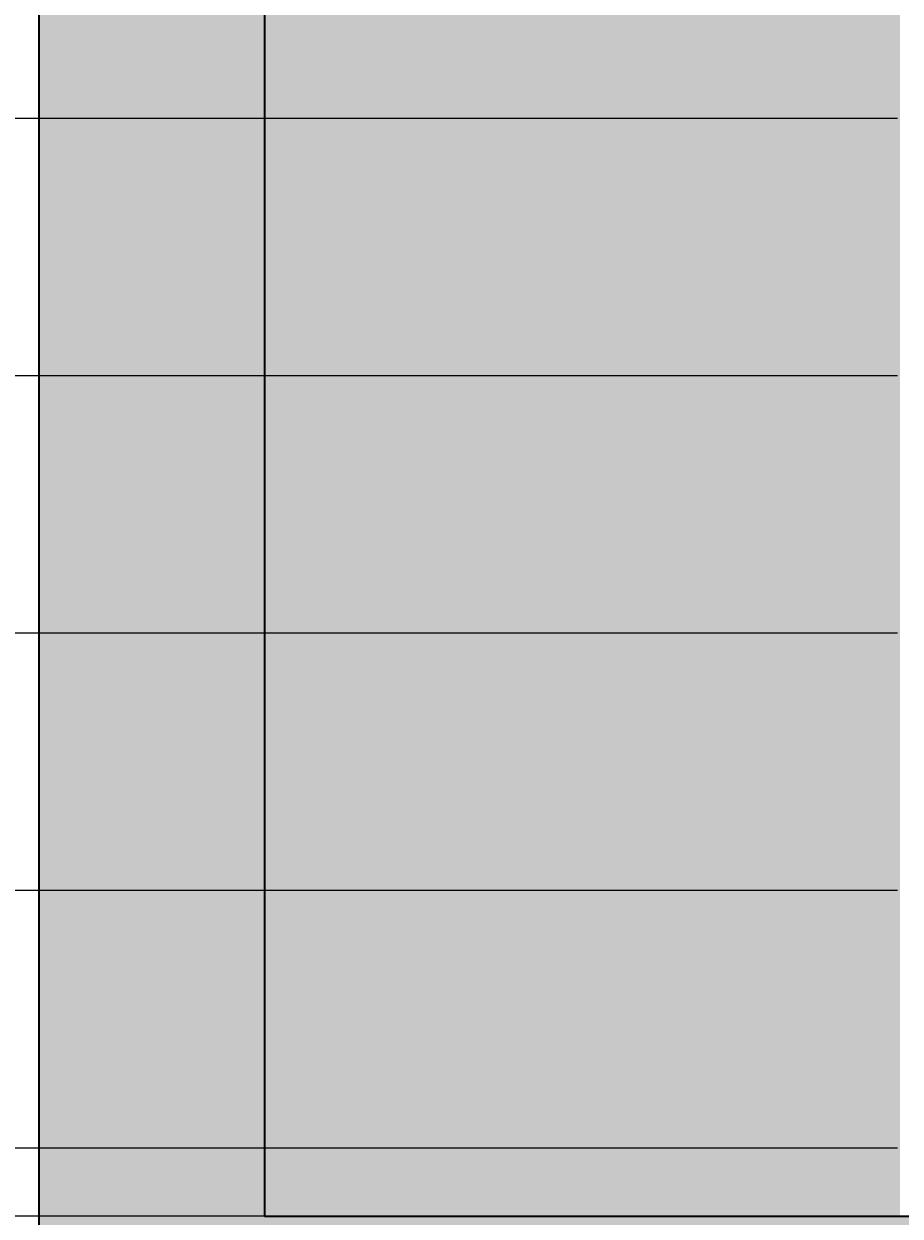
# Model space of a CAD drawing. Units: feet. Extents: x 2695 to 2912, y 795 to 1139.
# Tile 36 of 83: x 2710 to 2731, y 937 to 965. Entities that reach past the tile are written whole.
import ezdxf

# ---------------------------------------------------------------- set-up
doc = ezdxf.new("R2010")
doc.units = ezdxf.units.FT
for name, color, linetype, lineweight in [('A-ANNO-DIMS', 2, 'Continuous', 18), ('A-ELEV', 7, 'Continuous', 35), ('A-ELEV-PATT', 252, 'Continuous', 13)]:
    doc.layers.add(name, color=color, linetype=linetype, lineweight=lineweight)
doc.styles.get("Standard").update_dxf_attribs({"font": 'arial.ttf'})
doc.dimstyles.get("Standard").update_dxf_attribs({"dimtxt": 0.18, "dimasz": 0.18, "dimexe": 0.18, "dimexo": 0.0625, "dimgap": 0.09, "dimtad": 0, "dimtih": 1, "dimtoh": 1, "dimdec": 1, "dimzin": 0, "dimdsep": 46, "dimlunit": 3, "dimtxsty": 'Standard', "dimcen": 0.09, "dimadec": 0, "dimazin": 0, "dimtfac": 1, "dimtdec": 1, "dimtofl": 0, "dimtmove": 0, "dimatfit": 3, "dimfxl": 1, "dimtolj": 1, "dimtzin": 0, "dimarcsym": 0})

# ---------------------------------------------------------------- blocks, each defined once
blk = doc.blocks.new('*D12')
at = {"layer": 'A-ANNO-DIMS', "color": 0, "lineweight": -2, "transparency": 16777216}
for p, q in [((2710.574, 1122.931), (2694.681, 1122.931)), ((2694.861, 1122.751), (2694.861, 967.113)), ((2694.861, 811.111), (2694.861, 966.749)), ((2710.574, 810.931), (2694.681, 810.931))]:
    blk.add_line(p, q, dxfattribs=at)
at = {"layer": 'A-ANNO-DIMS', "color": 0, "transparency": 16777216}
for points in [[(2694.831, 1122.751), (2694.891, 1122.751), (2694.861, 1122.931)], [(2694.831, 811.111), (2694.891, 811.111), (2694.861, 810.931)]]:
    blk.add_solid(points, dxfattribs=at)
at = {"layer": 'Defpoints', "color": 0, "transparency": 16777216}
for p in [(2694.861, 1122.931), (2710.636, 1122.931), (2710.636, 810.931)]:
    blk.add_point(p, dxfattribs=at)
at = {"layer": 'A-ANNO-DIMS', "color": 0, "transparency": 16777216, "insert": (2694.861, 966.931), "char_height": 0.18, "attachment_point": 5}
blk.add_mtext('\\A1;312', dxfattribs=at)
blk = doc.blocks.new('*D27')
at = {"layer": 'A-ANNO-DIMS', "color": 0, "lineweight": -2, "transparency": 16777216}
for p, q in [((2730.646, 938.518), (2694.681, 938.518)), ((2694.861, 938.338), (2694.861, 937.906)), ((2694.861, 937.111), (2694.861, 937.542)), ((2730.646, 936.931), (2694.681, 936.931))]:
    blk.add_line(p, q, dxfattribs=at)
at = {"layer": 'A-ANNO-DIMS', "color": 0, "transparency": 16777216}
for points in [[(2694.831, 938.338), (2694.891, 938.338), (2694.861, 938.518)], [(2694.831, 937.111), (2694.891, 937.111), (2694.861, 936.931)]]:
    blk.add_solid(points, dxfattribs=at)
at = {"layer": 'Defpoints', "color": 0, "transparency": 16777216}
for p in [(2694.861, 938.518), (2730.708, 938.518), (2730.708, 936.931)]:
    blk.add_point(p, dxfattribs=at)
at = {"layer": 'A-ANNO-DIMS', "color": 0, "transparency": 16777216, "insert": (2694.861, 937.724), "char_height": 0.18, "attachment_point": 5}
blk.add_mtext('\\A1;1.59', dxfattribs=at)
blk = doc.blocks.new('*D28')
at = {"layer": 'A-ANNO-DIMS', "color": 0, "lineweight": -2, "transparency": 16777216}
for p, q in [((2730.646, 944.518), (2694.681, 944.518)), ((2694.861, 944.338), (2694.861, 941.7)), ((2694.861, 938.698), (2694.861, 941.336)), ((2730.646, 938.518), (2694.681, 938.518))]:
    blk.add_line(p, q, dxfattribs=at)
at = {"layer": 'A-ANNO-DIMS', "color": 0, "transparency": 16777216}
for points in [[(2694.831, 944.338), (2694.891, 944.338), (2694.861, 944.518)], [(2694.831, 938.698), (2694.891, 938.698), (2694.861, 938.518)]]:
    blk.add_solid(points, dxfattribs=at)
at = {"layer": 'Defpoints', "color": 0, "transparency": 16777216}
for p in [(2694.861, 944.518), (2730.708, 944.518), (2730.708, 938.518)]:
    blk.add_point(p, dxfattribs=at)
at = {"layer": 'A-ANNO-DIMS', "color": 0, "transparency": 16777216, "insert": (2694.861, 941.518), "char_height": 0.18, "attachment_point": 5}
blk.add_mtext('\\A1;6', dxfattribs=at)
blk = doc.blocks.new('*D29')
at = {"layer": 'A-ANNO-DIMS', "color": 0, "lineweight": -2, "transparency": 16777216}
for p, q in [((2730.646, 950.518), (2694.681, 950.518)), ((2694.861, 950.338), (2694.861, 947.7)), ((2694.861, 944.698), (2694.861, 947.336)), ((2730.646, 944.518), (2694.681, 944.518))]:
    blk.add_line(p, q, dxfattribs=at)
at = {"layer": 'A-ANNO-DIMS', "color": 0, "transparency": 16777216}
for points in [[(2694.831, 950.338), (2694.891, 950.338), (2694.861, 950.518)], [(2694.831, 944.698), (2694.891, 944.698), (2694.861, 944.518)]]:
    blk.add_solid(points, dxfattribs=at)
at = {"layer": 'Defpoints', "color": 0, "transparency": 16777216}
for p in [(2694.861, 950.518), (2730.708, 950.518), (2730.708, 944.518)]:
    blk.add_point(p, dxfattribs=at)
at = {"layer": 'A-ANNO-DIMS', "color": 0, "transparency": 16777216, "insert": (2694.861, 947.518), "char_height": 0.18, "attachment_point": 5}
blk.add_mtext('\\A1;6', dxfattribs=at)
blk = doc.blocks.new('*D30')
at = {"layer": 'A-ANNO-DIMS', "color": 0, "lineweight": -2, "transparency": 16777216}
for p, q in [((2730.646, 956.518), (2694.681, 956.518)), ((2694.861, 956.338), (2694.861, 953.7)), ((2694.861, 950.698), (2694.861, 953.336)), ((2730.646, 950.518), (2694.681, 950.518))]:
    blk.add_line(p, q, dxfattribs=at)
at = {"layer": 'A-ANNO-DIMS', "color": 0, "transparency": 16777216}
for points in [[(2694.831, 956.338), (2694.891, 956.338), (2694.861, 956.518)], [(2694.831, 950.698), (2694.891, 950.698), (2694.861, 950.518)]]:
    blk.add_solid(points, dxfattribs=at)
at = {"layer": 'Defpoints', "color": 0, "transparency": 16777216}
for p in [(2694.861, 956.518), (2730.708, 956.518), (2730.708, 950.518)]:
    blk.add_point(p, dxfattribs=at)
at = {"layer": 'A-ANNO-DIMS', "color": 0, "transparency": 16777216, "insert": (2694.861, 953.518), "char_height": 0.18, "attachment_point": 5}
blk.add_mtext('\\A1;6', dxfattribs=at)
blk = doc.blocks.new('*D31')
at = {"layer": 'A-ANNO-DIMS', "color": 0, "lineweight": -2, "transparency": 16777216}
for p, q in [((2730.646, 962.518), (2694.681, 962.518)), ((2694.861, 962.338), (2694.861, 959.7)), ((2694.861, 956.698), (2694.861, 959.336)), ((2730.646, 956.518), (2694.681, 956.518))]:
    blk.add_line(p, q, dxfattribs=at)
at = {"layer": 'A-ANNO-DIMS', "color": 0, "transparency": 16777216}
for points in [[(2694.831, 962.338), (2694.891, 962.338), (2694.861, 962.518)], [(2694.831, 956.698), (2694.891, 956.698), (2694.861, 956.518)]]:
    blk.add_solid(points, dxfattribs=at)
at = {"layer": 'Defpoints', "color": 0, "transparency": 16777216}
for p in [(2694.861, 962.518), (2730.708, 962.518), (2730.708, 956.518)]:
    blk.add_point(p, dxfattribs=at)
at = {"layer": 'A-ANNO-DIMS', "color": 0, "transparency": 16777216, "insert": (2694.861, 959.518), "char_height": 0.18, "attachment_point": 5}
blk.add_mtext('\\A1;6', dxfattribs=at)
blk = doc.blocks.new('*D32')
at = {"layer": 'A-ANNO-DIMS', "color": 0, "lineweight": -2, "transparency": 16777216}
for p, q in [((2730.646, 968.518), (2694.681, 968.518)), ((2694.861, 968.338), (2694.861, 965.7)), ((2694.861, 962.698), (2694.861, 965.336)), ((2730.646, 962.518), (2694.681, 962.518))]:
    blk.add_line(p, q, dxfattribs=at)
at = {"layer": 'A-ANNO-DIMS', "color": 0, "transparency": 16777216}
for points in [[(2694.831, 968.338), (2694.891, 968.338), (2694.861, 968.518)], [(2694.831, 962.698), (2694.891, 962.698), (2694.861, 962.518)]]:
    blk.add_solid(points, dxfattribs=at)
at = {"layer": 'Defpoints', "color": 0, "transparency": 16777216}
for p in [(2694.861, 968.518), (2730.708, 968.518), (2730.708, 962.518)]:
    blk.add_point(p, dxfattribs=at)
at = {"layer": 'A-ANNO-DIMS', "color": 0, "transparency": 16777216, "insert": (2694.861, 965.518), "char_height": 0.18, "attachment_point": 5}
blk.add_mtext('\\A1;6', dxfattribs=at)

msp = doc.modelspace()

# ---------------------------------------------------------------- hatches: boundary and pattern name
at = {"layer": 'A-ELEV-PATT'}
h = msp.add_hatch(color=256, dxfattribs=at)
h.set_gradient(color1=(255, 255, 255), tint=1)
h.paths.add_polyline_path([(2770.6361, 1122.9306), (2710.6361, 1122.9306), (2710.6361, 1118.4096), (2770.6361, 1118.4096)])
h.paths.add_polyline_path([(2890.6361, 1107.8588), (2770.6361, 1107.8588), (2770.6361, 1103.3378), (2890.6361, 1103.3378)])
h.paths.add_polyline_path([(2890.6361, 1062.9306), (2710.6361, 1062.9306), (2710.6361, 1056.9306), (2710.6361, 936.9306), (2710.6361, 924.3105), (2716.5358, 924.3105), (2890.6361, 924.3105), (2890.6361, 936.9306), (2715.8852, 936.9306), (2715.8852, 1050.3105), (2890.6361, 1050.3105)])
h.paths.add_polyline_path([(2716.5358, 924.3105), (2710.6361, 924.3105), (2710.6361, 810.9306), (2716.5358, 810.9306)])
h = msp.add_hatch(color=256, dxfattribs=at)
h.set_gradient(color1=(147, 149, 152), color2=(147, 149, 152), tint=1)
h.paths.add_polyline_path([(2770.6361, 1118.4096), (2710.6361, 1118.4096), (2710.6361, 1062.9306), (2770.6361, 1062.9306)])
h.paths.add_polyline_path([(2890.6361, 1103.3378), (2770.6361, 1103.3378), (2770.6361, 1062.9306), (2890.6361, 1062.9306)])
h.paths.add_polyline_path([(2730.7081, 1048.1052), (2755.1125, 1048.1052), (2755.1125, 936.9306), (2770.6361, 936.9306), (2770.6361, 1050.3105), (2715.8852, 1050.3105), (2715.8852, 936.9306), (2730.7081, 936.9306)])
h.paths.add_polyline_path([(2890.6361, 1050.3105), (2770.6361, 1050.3105), (2770.6361, 971.9673), (2778.0341, 971.9673), (2778.0341, 1020.8235), (2843.575, 1020.8235), (2843.575, 971.9673), (2890.6361, 971.9673)])
h.paths.add_polyline_path([(2888.1882, 970.7156), (2843.575, 970.7156), (2843.575, 964.8267), (2888.1882, 964.8267)])
h.paths.add_polyline_path([(2888.1882, 964.1328), (2843.575, 964.1328), (2843.575, 956.614), (2888.1882, 956.614)])
h.paths.add_polyline_path([(2888.1882, 955.9202), (2843.575, 955.9202), (2843.575, 949.2892), (2888.1882, 949.2892)])
h.paths.add_polyline_path([(2888.1882, 948.5954), (2843.575, 948.5954), (2843.575, 941.3507), (2888.1882, 941.3507)])
h.paths.add_polyline_path([(2888.1882, 940.6569), (2843.575, 940.6569), (2843.575, 936.9306), (2888.1882, 936.9306)])
h.paths.add_polyline_path([(2890.6361, 970.7156), (2888.9368, 970.7156), (2888.9368, 964.8267), (2890.6361, 964.8267)])
h.paths.add_polyline_path([(2890.6361, 964.1328), (2888.9368, 964.1328), (2888.9368, 956.614), (2890.6361, 956.614)])
h.paths.add_polyline_path([(2890.6361, 955.9202), (2888.9368, 955.9202), (2888.9368, 949.2892), (2890.6361, 949.2892)])
h.paths.add_polyline_path([(2890.6361, 940.6569), (2888.9368, 940.6569), (2888.9368, 936.9306), (2890.6361, 936.9306)])
h.paths.add_polyline_path([(2890.6361, 948.5954), (2888.9368, 948.5954), (2888.9368, 941.3507), (2890.6361, 941.3507)])
h.paths.add_polyline_path([(2772.5216, 970.7156), (2770.6361, 970.7156), (2770.6361, 964.8267), (2772.5216, 964.8267)])
h.paths.add_polyline_path([(2772.5216, 964.1328), (2770.6361, 964.1328), (2770.6361, 956.614), (2772.5216, 956.614)])
h.paths.add_polyline_path([(2772.5216, 955.9202), (2770.6361, 955.9202), (2770.6361, 949.2892), (2772.5216, 949.2892)])
h.paths.add_polyline_path([(2772.5216, 948.5954), (2770.6361, 948.5954), (2770.6361, 941.3507), (2772.5216, 941.3507)])
h.paths.add_polyline_path([(2772.5216, 940.6569), (2770.6361, 940.6569), (2770.6361, 936.9306), (2772.5216, 936.9306)])
h.paths.add_polyline_path([(2778.0341, 940.6569), (2773.2702, 940.6569), (2773.2702, 936.9306), (2778.0341, 936.9306)])
h.paths.add_polyline_path([(2778.0341, 970.7156), (2773.2702, 970.7156), (2773.2702, 964.8267), (2778.0341, 964.8267)])
h.paths.add_polyline_path([(2778.0341, 964.1328), (2773.2702, 964.1328), (2773.2702, 956.614), (2778.0341, 956.614)])
h.paths.add_polyline_path([(2778.0341, 955.9202), (2773.2702, 955.9202), (2773.2702, 949.2892), (2778.0341, 949.2892)])
h.paths.add_polyline_path([(2778.0341, 948.5954), (2773.2702, 948.5954), (2773.2702, 941.3507), (2778.0341, 941.3507)])
h.paths.add_polyline_path([(2810.0407, 940.6569), (2780.0341, 940.6569), (2780.0341, 936.9306), (2810.0407, 936.9306)])
h.paths.add_polyline_path([(2890.6361, 924.3105), (2770.6361, 924.3105), (2770.6361, 810.9306), (2773.5029, 810.9306), (2773.5029, 905.5143), (2805.9398, 905.5143), (2838.3767, 905.5143), (2838.3767, 810.9306), (2890.6361, 810.9306)])

# ---------------------------------------------------------------- linework, layer by layer
at = {"layer": 'A-ELEV'}
for p, q in [((2710.6361, 936.9306), (2710.6361, 1056.9306)), ((2715.8852, 1050.3105), (2715.8852, 936.9306)), ((2710.6361, 930.9306), (2710.6361, 936.9306)), ((2715.8852, 936.9306), (2890.6361, 936.9306)), ((2715.8852, 936.9306), (2890.6361, 936.9306))]:
    msp.add_line(p, q, dxfattribs=at)
for points in [[(2715.8852, 1050.3105), (2715.8852, 936.9306)], [(2890.6361, 936.9306), (2890.6361, 924.3105), (2710.6361, 924.3105), (2710.6361, 936.9306)]]:
    msp.add_lwpolyline(points, dxfattribs=at)

# ---------------------------------------------------------------- dimensions: what is measured, and where the dimension line sits
at = {"layer": 'A-ANNO-DIMS'}
for base, p1, p2, override, picture, middle in [((2694.8611, 1122.9306), (2710.6361, 810.9306), (2710.6361, 1122.9306), {"dimdec": 0, "dimlfac": 1, "dimrnd": 0, "dimzin": 0, "dimdsep": 46, "dimlunit": 2}, '*D12', (2694.8611, 966.9306)), ((2694.8611, 968.5179), (2730.7081, 962.5179), (2730.7081, 968.5179), {"dimdec": 0, "dimlfac": 1, "dimrnd": 0, "dimzin": 0, "dimdsep": 46, "dimlunit": 2}, '*D32', (2694.8611, 965.5179)), ((2694.8611, 962.5179), (2730.7081, 956.5179), (2730.7081, 962.5179), {"dimdec": 0, "dimlfac": 1, "dimrnd": 0, "dimzin": 0, "dimdsep": 46, "dimlunit": 2}, '*D31', (2694.8611, 959.5179)), ((2694.8611, 956.5179), (2730.7081, 950.5179), (2730.7081, 956.5179), {"dimdec": 0, "dimlfac": 1, "dimrnd": 0, "dimzin": 0, "dimdsep": 46, "dimlunit": 2}, '*D30', (2694.8611, 953.5179)), ((2694.8611, 950.5179), (2730.7081, 944.5179), (2730.7081, 950.5179), {"dimdec": 0, "dimlfac": 1, "dimrnd": 0, "dimzin": 0, "dimdsep": 46, "dimlunit": 2}, '*D29', (2694.8611, 947.5179)), ((2694.8611, 944.5179), (2730.7081, 938.5179), (2730.7081, 944.5179), {"dimdec": 0, "dimlfac": 1, "dimrnd": 0, "dimzin": 0, "dimdsep": 46, "dimlunit": 2}, '*D28', (2694.8611, 941.5179)), ((2694.8611, 938.5179), (2730.7081, 936.9306), (2730.7081, 938.5179), {"dimdec": 2, "dimlfac": 1, "dimrnd": 0, "dimzin": 0, "dimdsep": 46, "dimlunit": 2}, '*D27', (2694.8611, 937.7242))]:
    dim = msp.add_linear_dim(base=base, p1=p1, p2=p2, angle=90, dimstyle='Standard', override=override, dxfattribs=at)
    dim.commit()
    dim.dimension.update_dxf_attribs({"geometry": picture, "text_midpoint": middle})

doc.saveas('drawing.dxf')
